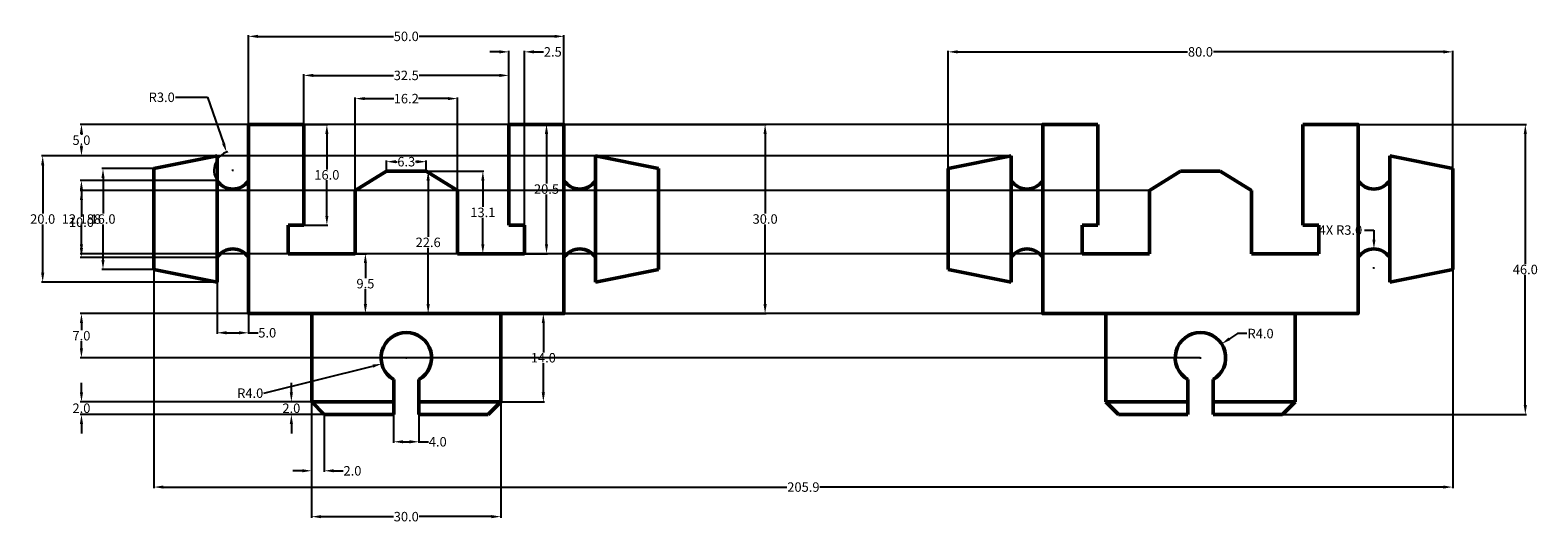
# Model space of a CAD drawing. Units: millimetres. Extents: x 10 to 249, y 5 to 83.
import ezdxf

# ---------------------------------------------------------------- set-up
doc = ezdxf.new("R2010")
doc.units = ezdxf.units.MM
doc.header["$MEASUREMENT"] = 0
doc.layers.add('M-DIMS', color=3, linetype='Continuous', lineweight=25)
doc.layers.add('M-OUTL', color=7, linetype='Continuous', lineweight=50)
doc.styles.get("Standard").update_dxf_attribs({"font": 'arial.ttf'})
doc.dimstyles.get("Standard").update_dxf_attribs({"dimtxt": 1.5, "dimasz": 1.5, "dimexe": 0.18, "dimexo": 0.0625, "dimgap": 0.09, "dimtad": 0, "dimtih": 1, "dimtoh": 1, "dimdec": 1, "dimzin": 0, "dimdsep": 46, "dimtxsty": 'Standard', "dimcen": 0.09, "dimadec": 0, "dimazin": 0, "dimtfac": 1, "dimtdec": 1, "dimtofl": 0, "dimtmove": 0, "dimatfit": 3, "dimfxl": 1, "dimtolj": 1, "dimtzin": 0, "dimarcsym": 0})

# ---------------------------------------------------------------- blocks, each defined once
blk = doc.blocks.new('*D1')
at = {"layer": 'Defpoints', "color": 0, "transparency": 16777216}
for p in [(66.62, 60.41), (72.92, 61.9), (72.92, 60.41)]:
    blk.add_point(p, dxfattribs=at)
at = {"layer": 'M-DIMS', "color": 0, "lineweight": -2, "transparency": 16777216}
for p, q in [((66.62, 60.47), (66.62, 62.08)), ((68.12, 61.9), (68.31, 61.9)), ((71.42, 61.9), (71.23, 61.9)), ((72.92, 60.47), (72.92, 62.08))]:
    blk.add_line(p, q, dxfattribs=at)
at = {"layer": 'M-DIMS', "color": 0, "transparency": 16777216}
for points in [[(68.12, 62.15), (68.12, 61.65), (66.62, 61.9)], [(71.42, 62.15), (71.42, 61.65), (72.92, 61.9)]]:
    blk.add_solid(points, dxfattribs=at)
at = {"layer": 'M-DIMS', "color": 0, "transparency": 16777216, "insert": (69.77, 61.9), "char_height": 1.5, "attachment_point": 5}
blk.add_mtext('\\A1;6.3', dxfattribs=at)
blk = doc.blocks.new('*D2')
at = {"layer": 'Defpoints', "color": 0, "transparency": 16777216}
for p in [(29.77, 60.81), (21.69, 44.81), (29.77, 44.81)]:
    blk.add_point(p, dxfattribs=at)
at = {"layer": 'M-DIMS', "color": 0, "lineweight": -2, "transparency": 16777216}
for p, q in [((29.71, 60.81), (21.51, 60.81)), ((21.69, 59.31), (21.69, 53.67)), ((21.69, 46.31), (21.69, 51.96)), ((29.71, 44.81), (21.51, 44.81))]:
    blk.add_line(p, q, dxfattribs=at)
at = {"layer": 'M-DIMS', "color": 0, "transparency": 16777216}
for points in [[(21.44, 59.31), (21.94, 59.31), (21.69, 60.81)], [(21.44, 46.31), (21.94, 46.31), (21.69, 44.81)]]:
    blk.add_solid(points, dxfattribs=at)
at = {"layer": 'M-DIMS', "color": 0, "transparency": 16777216, "insert": (21.69, 52.81), "char_height": 1.5, "attachment_point": 5}
blk.add_mtext('\\A1;16.0', dxfattribs=at)
blk = doc.blocks.new('*D3')
at = {"layer": 'Defpoints', "color": 0, "transparency": 16777216}
for p in [(39.77, 62.81), (12.13, 42.81), (39.77, 42.81)]:
    blk.add_point(p, dxfattribs=at)
at = {"layer": 'M-DIMS', "color": 0, "lineweight": -2, "transparency": 16777216}
for p, q in [((39.71, 62.81), (11.95, 62.81)), ((12.13, 61.31), (12.13, 53.67)), ((12.13, 44.31), (12.13, 51.96)), ((39.71, 42.81), (11.95, 42.81))]:
    blk.add_line(p, q, dxfattribs=at)
at = {"layer": 'M-DIMS', "color": 0, "transparency": 16777216}
for points in [[(11.88, 61.31), (12.38, 61.31), (12.13, 62.81)], [(11.88, 44.31), (12.38, 44.31), (12.13, 42.81)]]:
    blk.add_solid(points, dxfattribs=at)
at = {"layer": 'M-DIMS', "color": 0, "transparency": 16777216, "insert": (12.13, 52.81), "char_height": 1.5, "attachment_point": 5}
blk.add_mtext('\\A1;20.0', dxfattribs=at)
blk = doc.blocks.new('*D4')
at = {"layer": 'Defpoints', "color": 0, "transparency": 16777216}
for p in [(41.29, 63.4), (42.27, 60.56)]:
    blk.add_point(p, dxfattribs=at)
at = {"layer": 'M-DIMS', "color": 0, "lineweight": -2, "transparency": 16777216}
for p, q in [((33.17, 72.11), (38.25, 72.11)), ((38.25, 72.11), (40.79, 64.81)), ((42.18, 60.56), (42.36, 60.56)), ((42.27, 60.47), (42.27, 60.65))]:
    blk.add_line(p, q, dxfattribs=at)
blk.add_arc((42.27, 60.56), 3, 105.7509, 212.3636, dxfattribs=at)
at = {"layer": 'M-DIMS', "color": 0, "transparency": 16777216}
blk.add_solid([(41.03, 64.9), (40.56, 64.73), (41.29, 63.4)], dxfattribs=at)
at = {"layer": 'M-DIMS', "color": 0, "transparency": 16777216, "insert": (31, 72.11), "char_height": 1.5, "attachment_point": 5}
blk.add_mtext('\\A1;R3.0', dxfattribs=at)
blk = doc.blocks.new('*D5')
at = {"layer": 'Defpoints', "color": 0, "transparency": 16777216}
for p in [(39.77, 42.81), (44.77, 42.81), (44.77, 34.77)]:
    blk.add_point(p, dxfattribs=at)
at = {"layer": 'M-DIMS', "color": 0, "lineweight": -2, "transparency": 16777216}
for p, q in [((39.77, 42.75), (39.77, 34.59)), ((44.77, 42.75), (44.77, 34.59)), ((41.27, 34.77), (43.27, 34.77)), ((44.77, 34.77), (46.27, 34.77))]:
    blk.add_line(p, q, dxfattribs=at)
at = {"layer": 'M-DIMS', "color": 0, "transparency": 16777216}
for points in [[(41.27, 35.02), (41.27, 34.52), (39.77, 34.77)], [(43.27, 35.02), (43.27, 34.52), (44.77, 34.77)]]:
    blk.add_solid(points, dxfattribs=at)
at = {"layer": 'M-DIMS', "color": 0, "transparency": 16777216, "insert": (47.73, 34.77), "char_height": 1.5, "attachment_point": 5}
blk.add_mtext('\\A1;5.0', dxfattribs=at)
blk = doc.blocks.new('*D6')
at = {"layer": 'Defpoints', "color": 0, "transparency": 16777216}
for p in [(65.89, 29.85), (69.77, 30.81)]:
    blk.add_point(p, dxfattribs=at)
at = {"layer": 'M-DIMS', "color": 0, "lineweight": -2, "transparency": 16777216}
for p, q in [((47.2, 25.2), (64.44, 29.48)), ((69.68, 30.81), (69.86, 30.81)), ((69.77, 30.72), (69.77, 30.9))]:
    blk.add_line(p, q, dxfattribs=at)
at = {"layer": 'M-DIMS', "color": 0, "transparency": 16777216}
blk.add_solid([(64.38, 29.73), (64.5, 29.24), (65.89, 29.85)], dxfattribs=at)
at = {"layer": 'M-DIMS', "color": 0, "transparency": 16777216, "insert": (45.03, 25.2), "char_height": 1.5, "attachment_point": 5}
blk.add_mtext('\\A1;R4.0', dxfattribs=at)
blk = doc.blocks.new('*D7')
at = {"layer": 'Defpoints', "color": 0, "transparency": 16777216}
for p in [(54.77, 23.81), (56.77, 21.81), (56.77, 12.89)]:
    blk.add_point(p, dxfattribs=at)
at = {"layer": 'M-DIMS', "color": 0, "lineweight": -2, "transparency": 16777216}
for p, q in [((54.77, 23.75), (54.77, 12.71)), ((56.77, 21.75), (56.77, 12.71)), ((53.27, 12.89), (51.77, 12.89)), ((58.27, 12.89), (59.77, 12.89))]:
    blk.add_line(p, q, dxfattribs=at)
at = {"layer": 'M-DIMS', "color": 0, "transparency": 16777216}
for points in [[(53.27, 13.14), (53.27, 12.64), (54.77, 12.89)], [(58.27, 13.14), (58.27, 12.64), (56.77, 12.89)]]:
    blk.add_solid(points, dxfattribs=at)
at = {"layer": 'M-DIMS', "color": 0, "transparency": 16777216, "insert": (61.24, 12.89), "char_height": 1.5, "attachment_point": 5}
blk.add_mtext('\\A1;2.0', dxfattribs=at)
blk = doc.blocks.new('*D8')
at = {"layer": 'Defpoints', "color": 0, "transparency": 16777216}
for p in [(51.55, 23.81), (54.77, 23.81), (56.77, 21.81)]:
    blk.add_point(p, dxfattribs=at)
at = {"layer": 'M-DIMS', "color": 0, "lineweight": -2, "transparency": 16777216}
for p, q in [((51.55, 25.31), (51.55, 26.81)), ((54.71, 23.81), (51.37, 23.81)), ((56.71, 21.81), (51.37, 21.81)), ((51.55, 20.31), (51.55, 18.81))]:
    blk.add_line(p, q, dxfattribs=at)
at = {"layer": 'M-DIMS', "color": 0, "transparency": 16777216}
for points in [[(51.3, 25.31), (51.8, 25.31), (51.55, 23.81)], [(51.3, 20.31), (51.8, 20.31), (51.55, 21.81)]]:
    blk.add_solid(points, dxfattribs=at)
at = {"layer": 'M-DIMS', "color": 0, "transparency": 16777216, "insert": (51.55, 22.81), "char_height": 1.5, "attachment_point": 5}
blk.add_mtext('\\A1;2.0', dxfattribs=at)
blk = doc.blocks.new('*D9')
at = {"layer": 'Defpoints', "color": 0, "transparency": 16777216}
for p in [(54.77, 23.81), (84.77, 23.81), (84.77, 5.62)]:
    blk.add_point(p, dxfattribs=at)
at = {"layer": 'M-DIMS', "color": 0, "lineweight": -2, "transparency": 16777216}
for p, q in [((54.77, 23.75), (54.77, 5.44)), ((84.77, 23.75), (84.77, 5.44)), ((56.27, 5.62), (67.74, 5.62)), ((83.27, 5.62), (71.81, 5.62))]:
    blk.add_line(p, q, dxfattribs=at)
at = {"layer": 'M-DIMS', "color": 0, "transparency": 16777216}
for points in [[(56.27, 5.87), (56.27, 5.37), (54.77, 5.62)], [(83.27, 5.87), (83.27, 5.37), (84.77, 5.62)]]:
    blk.add_solid(points, dxfattribs=at)
at = {"layer": 'M-DIMS', "color": 0, "transparency": 16777216, "insert": (69.77, 5.62), "char_height": 1.5, "attachment_point": 5}
blk.add_mtext('\\A1;30.0', dxfattribs=at)
blk = doc.blocks.new('*D10')
at = {"layer": 'Defpoints', "color": 0, "transparency": 16777216}
for p in [(67.77, 21.81), (71.77, 21.81), (71.77, 17.49)]:
    blk.add_point(p, dxfattribs=at)
at = {"layer": 'M-DIMS', "color": 0, "lineweight": -2, "transparency": 16777216}
for p, q in [((67.77, 21.75), (67.77, 17.31)), ((71.77, 21.75), (71.77, 17.31)), ((69.27, 17.49), (70.27, 17.49)), ((71.77, 17.49), (73.27, 17.49))]:
    blk.add_line(p, q, dxfattribs=at)
at = {"layer": 'M-DIMS', "color": 0, "transparency": 16777216}
for points in [[(69.27, 17.74), (69.27, 17.24), (67.77, 17.49)], [(70.27, 17.74), (70.27, 17.24), (71.77, 17.49)]]:
    blk.add_solid(points, dxfattribs=at)
at = {"layer": 'M-DIMS', "color": 0, "transparency": 16777216, "insert": (74.76, 17.49), "char_height": 1.5, "attachment_point": 5}
blk.add_mtext('\\A1;4.0', dxfattribs=at)
blk = doc.blocks.new('*D11')
at = {"layer": 'Defpoints', "color": 0, "transparency": 16777216}
for p in [(84.77, 37.81), (91.5, 37.81), (84.77, 23.81)]:
    blk.add_point(p, dxfattribs=at)
at = {"layer": 'M-DIMS', "color": 0, "lineweight": -2, "transparency": 16777216}
for p, q in [((84.84, 37.81), (91.68, 37.81)), ((91.5, 36.31), (91.5, 31.67)), ((91.5, 25.31), (91.5, 29.96)), ((84.84, 23.81), (91.68, 23.81))]:
    blk.add_line(p, q, dxfattribs=at)
at = {"layer": 'M-DIMS', "color": 0, "transparency": 16777216}
for points in [[(91.25, 36.31), (91.75, 36.31), (91.5, 37.81)], [(91.25, 25.31), (91.75, 25.31), (91.5, 23.81)]]:
    blk.add_solid(points, dxfattribs=at)
at = {"layer": 'M-DIMS', "color": 0, "transparency": 16777216, "insert": (91.5, 30.81), "char_height": 1.5, "attachment_point": 5}
blk.add_mtext('\\A1;14.0', dxfattribs=at)
blk = doc.blocks.new('*D12')
at = {"layer": 'Defpoints', "color": 0, "transparency": 16777216}
for p in [(94.77, 67.81), (126.66, 67.81), (94.77, 37.81)]:
    blk.add_point(p, dxfattribs=at)
at = {"layer": 'M-DIMS', "color": 0, "lineweight": -2, "transparency": 16777216}
for p, q in [((94.84, 67.81), (126.84, 67.81)), ((126.66, 66.31), (126.66, 53.67)), ((126.66, 39.31), (126.66, 51.96)), ((94.84, 37.81), (126.84, 37.81))]:
    blk.add_line(p, q, dxfattribs=at)
at = {"layer": 'M-DIMS', "color": 0, "transparency": 16777216}
for points in [[(126.41, 66.31), (126.91, 66.31), (126.66, 67.81)], [(126.41, 39.31), (126.91, 39.31), (126.66, 37.81)]]:
    blk.add_solid(points, dxfattribs=at)
at = {"layer": 'M-DIMS', "color": 0, "transparency": 16777216, "insert": (126.66, 52.81), "char_height": 1.5, "attachment_point": 5}
blk.add_mtext('\\A1;30.0', dxfattribs=at)
blk = doc.blocks.new('*D13')
at = {"layer": 'Defpoints', "color": 0, "transparency": 16777216}
for p in [(94.77, 81.77), (44.77, 67.81), (94.77, 67.81)]:
    blk.add_point(p, dxfattribs=at)
at = {"layer": 'M-DIMS', "color": 0, "lineweight": -2, "transparency": 16777216}
for p, q in [((44.77, 67.87), (44.77, 81.95)), ((46.27, 81.77), (67.74, 81.77)), ((93.27, 81.77), (71.81, 81.77)), ((94.77, 67.87), (94.77, 81.95))]:
    blk.add_line(p, q, dxfattribs=at)
at = {"layer": 'M-DIMS', "color": 0, "transparency": 16777216}
for points in [[(46.27, 82.02), (46.27, 81.52), (44.77, 81.77)], [(93.27, 82.02), (93.27, 81.52), (94.77, 81.77)]]:
    blk.add_solid(points, dxfattribs=at)
at = {"layer": 'M-DIMS', "color": 0, "transparency": 16777216, "insert": (69.77, 81.77), "char_height": 1.5, "attachment_point": 5}
blk.add_mtext('\\A1;50.0', dxfattribs=at)
blk = doc.blocks.new('*D14')
at = {"layer": 'Defpoints', "color": 0, "transparency": 16777216}
for p in [(86.02, 75.58), (53.52, 67.81), (86.02, 67.81)]:
    blk.add_point(p, dxfattribs=at)
at = {"layer": 'M-DIMS', "color": 0, "lineweight": -2, "transparency": 16777216}
for p, q in [((53.52, 67.87), (53.52, 75.76)), ((55.02, 75.58), (67.73, 75.58)), ((84.52, 75.58), (71.82, 75.58)), ((86.02, 67.87), (86.02, 75.76))]:
    blk.add_line(p, q, dxfattribs=at)
at = {"layer": 'M-DIMS', "color": 0, "transparency": 16777216}
for points in [[(55.02, 75.83), (55.02, 75.33), (53.52, 75.58)], [(84.52, 75.83), (84.52, 75.33), (86.02, 75.58)]]:
    blk.add_solid(points, dxfattribs=at)
at = {"layer": 'M-DIMS', "color": 0, "transparency": 16777216, "insert": (69.77, 75.58), "char_height": 1.5, "attachment_point": 5}
blk.add_mtext('\\A1;32.5', dxfattribs=at)
blk = doc.blocks.new('*D15')
at = {"layer": 'Defpoints', "color": 0, "transparency": 16777216}
for p in [(77.87, 71.9), (61.67, 57.31), (77.87, 57.31)]:
    blk.add_point(p, dxfattribs=at)
at = {"layer": 'M-DIMS', "color": 0, "lineweight": -2, "transparency": 16777216}
for p, q in [((61.67, 57.37), (61.67, 72.08)), ((63.17, 71.9), (67.81, 71.9)), ((76.37, 71.9), (71.73, 71.9)), ((77.87, 57.37), (77.87, 72.08))]:
    blk.add_line(p, q, dxfattribs=at)
at = {"layer": 'M-DIMS', "color": 0, "transparency": 16777216}
for points in [[(63.17, 72.15), (63.17, 71.65), (61.67, 71.9)], [(76.37, 72.15), (76.37, 71.65), (77.87, 71.9)]]:
    blk.add_solid(points, dxfattribs=at)
at = {"layer": 'M-DIMS', "color": 0, "transparency": 16777216, "insert": (69.77, 71.9), "char_height": 1.5, "attachment_point": 5}
blk.add_mtext('\\A1;16.2', dxfattribs=at)
blk = doc.blocks.new('*D16')
at = {"layer": 'Defpoints', "color": 0, "transparency": 16777216}
for p in [(53.52, 67.81), (53.52, 51.81), (57.18, 51.81)]:
    blk.add_point(p, dxfattribs=at)
at = {"layer": 'M-DIMS', "color": 0, "lineweight": -2, "transparency": 16777216}
for p, q in [((53.59, 67.81), (57.36, 67.81)), ((57.18, 66.31), (57.18, 60.67)), ((57.18, 53.31), (57.18, 58.96)), ((53.59, 51.81), (57.36, 51.81))]:
    blk.add_line(p, q, dxfattribs=at)
at = {"layer": 'M-DIMS', "color": 0, "transparency": 16777216}
for points in [[(56.93, 66.31), (57.43, 66.31), (57.18, 67.81)], [(56.93, 53.31), (57.43, 53.31), (57.18, 51.81)]]:
    blk.add_solid(points, dxfattribs=at)
at = {"layer": 'M-DIMS', "color": 0, "transparency": 16777216, "insert": (57.18, 59.81), "char_height": 1.5, "attachment_point": 5}
blk.add_mtext('\\A1;16.0', dxfattribs=at)
blk = doc.blocks.new('*D17')
at = {"layer": 'Defpoints', "color": 0, "transparency": 16777216}
for p in [(61.67, 47.31), (61.67, 37.81), (63.29, 37.81)]:
    blk.add_point(p, dxfattribs=at)
at = {"layer": 'M-DIMS', "color": 0, "lineweight": -2, "transparency": 16777216}
for p, q in [((61.74, 47.31), (63.47, 47.31)), ((63.29, 45.81), (63.29, 43.42)), ((63.29, 39.31), (63.29, 41.71)), ((61.74, 37.81), (63.47, 37.81))]:
    blk.add_line(p, q, dxfattribs=at)
at = {"layer": 'M-DIMS', "color": 0, "transparency": 16777216}
for points in [[(63.04, 45.81), (63.54, 45.81), (63.29, 47.31)], [(63.04, 39.31), (63.54, 39.31), (63.29, 37.81)]]:
    blk.add_solid(points, dxfattribs=at)
at = {"layer": 'M-DIMS', "color": 0, "transparency": 16777216, "insert": (63.29, 42.56), "char_height": 1.5, "attachment_point": 5}
blk.add_mtext('\\A1;9.5', dxfattribs=at)
blk = doc.blocks.new('*D18')
at = {"layer": 'Defpoints', "color": 0, "transparency": 16777216}
for p in [(72.92, 60.41), (72.92, 37.81), (73.24, 37.81)]:
    blk.add_point(p, dxfattribs=at)
at = {"layer": 'M-DIMS', "color": 0, "lineweight": -2, "transparency": 16777216}
for p, q in [((72.99, 60.41), (73.42, 60.41)), ((73.24, 58.91), (73.24, 49.97)), ((73.24, 39.31), (73.24, 48.26)), ((72.99, 37.81), (73.42, 37.81))]:
    blk.add_line(p, q, dxfattribs=at)
at = {"layer": 'M-DIMS', "color": 0, "transparency": 16777216}
for points in [[(72.99, 58.91), (73.49, 58.91), (73.24, 60.41)], [(72.99, 39.31), (73.49, 39.31), (73.24, 37.81)]]:
    blk.add_solid(points, dxfattribs=at)
at = {"layer": 'M-DIMS', "color": 0, "transparency": 16777216, "insert": (73.24, 49.11), "char_height": 1.5, "attachment_point": 5}
blk.add_mtext('\\A1;22.6', dxfattribs=at)
blk = doc.blocks.new('*D19')
at = {"layer": 'Defpoints', "color": 0, "transparency": 16777216}
for p in [(72.92, 60.41), (77.87, 47.31), (81.91, 47.31)]:
    blk.add_point(p, dxfattribs=at)
at = {"layer": 'M-DIMS', "color": 0, "lineweight": -2, "transparency": 16777216}
for p, q in [((72.99, 60.41), (82.09, 60.41)), ((81.91, 58.91), (81.91, 54.72)), ((81.91, 48.81), (81.91, 53.01)), ((77.94, 47.31), (82.09, 47.31))]:
    blk.add_line(p, q, dxfattribs=at)
at = {"layer": 'M-DIMS', "color": 0, "transparency": 16777216}
for points in [[(81.66, 58.91), (82.16, 58.91), (81.91, 60.41)], [(81.66, 48.81), (82.16, 48.81), (81.91, 47.31)]]:
    blk.add_solid(points, dxfattribs=at)
at = {"layer": 'M-DIMS', "color": 0, "transparency": 16777216, "insert": (81.91, 53.86), "char_height": 1.5, "attachment_point": 5}
blk.add_mtext('\\A1;13.1', dxfattribs=at)
blk = doc.blocks.new('*D20')
at = {"layer": 'Defpoints', "color": 0, "transparency": 16777216}
for p in [(86.02, 67.81), (92, 67.81), (88.52, 47.31)]:
    blk.add_point(p, dxfattribs=at)
at = {"layer": 'M-DIMS', "color": 0, "lineweight": -2, "transparency": 16777216}
for p, q in [((86.09, 67.81), (92.18, 67.81)), ((92, 66.31), (92, 58.42)), ((92, 48.81), (92, 56.71)), ((88.59, 47.31), (92.18, 47.31))]:
    blk.add_line(p, q, dxfattribs=at)
at = {"layer": 'M-DIMS', "color": 0, "transparency": 16777216}
for points in [[(91.75, 66.31), (92.25, 66.31), (92, 67.81)], [(91.75, 48.81), (92.25, 48.81), (92, 47.31)]]:
    blk.add_solid(points, dxfattribs=at)
at = {"layer": 'M-DIMS', "color": 0, "transparency": 16777216, "insert": (92, 57.56), "char_height": 1.5, "attachment_point": 5}
blk.add_mtext('\\A1;20.5', dxfattribs=at)
blk = doc.blocks.new('MOUNTING-BRACKET-PROFILE')
for p, q in [((-16.25, 30), (-16.25, 14)), ((16.25, 30), (16.25, 14)), ((-40, 23), (-30, 25)), ((-30, 25), (-30, 5)), ((30, 25), (30, 5)), ((40, 23), (30, 25)), ((-40, 23), (-40, 7)), ((-8.1, 19.5), (-3.15, 22.6)), ((-3.15, 22.6), (3.15, 22.6)), ((8.1, 19.5), (3.15, 22.6)), ((40, 23), (40, 7)), ((-8.1, 9.5), (-8.1, 19.5)), ((8.1, 9.5), (8.1, 19.5)), ((-16.25, 14), (-18.75, 14)), ((-18.75, 14), (-18.75, 9.5)), ((16.25, 14), (18.75, 14)), ((18.75, 14), (18.75, 9.5)), ((-18.75, 9.5), (-8.1, 9.5)), ((8.1, 9.5), (18.75, 9.5)), ((-40, 7), (-30, 5)), ((40, 7), (30, 5)), ((-15, -14), (-15, 0)), ((-15, 0), (15, 0)), ((15, 0), (15, -14)), ((-2, -16), (-2, -10.46)), ((2, -16), (2, -10.46)), ((-15, -14), (-2, -14)), ((-13, -16), (-15, -14)), ((2, -14), (15, -14)), ((13, -16), (15, -14)), ((-13, -16), (-2, -16)), ((2, -16), (13, -16))]:
    blk.add_line(p, q)
blk.add_lwpolyline([(16.25, 30), (25, 30), (25, 0), (-25, 0), (-25, 30), (-16.25, 30)])
for centre, radius, start, end in [((-27.5, 22.75), 3, 213.5573, 326.4427), ((27.5, 22.75), 3, 213.5573, 326.4427), ((-27.5, 7.25), 3, 33.5573, 146.4427), ((27.5, 7.25), 3, 33.5573, 146.4427), ((0, -7), 4, 300, 240)]:
    blk.add_arc(centre, radius, start, end)
blk = doc.blocks.new('*D22')
at = {"layer": 'Defpoints', "color": 0, "transparency": 16777216}
for p in [(29.77, 44.81), (235.68, 44.81), (235.68, 10.31)]:
    blk.add_point(p, dxfattribs=at)
at = {"layer": 'M-DIMS', "color": 0, "lineweight": -2, "transparency": 16777216}
for p, q in [((29.77, 44.75), (29.77, 10.13)), ((235.68, 44.75), (235.68, 10.13)), ((31.27, 10.31), (130.09, 10.31)), ((234.18, 10.31), (135.36, 10.31))]:
    blk.add_line(p, q, dxfattribs=at)
at = {"layer": 'M-DIMS', "color": 0, "transparency": 16777216}
for points in [[(31.27, 10.56), (31.27, 10.06), (29.77, 10.31)], [(234.18, 10.56), (234.18, 10.06), (235.68, 10.31)]]:
    blk.add_solid(points, dxfattribs=at)
at = {"layer": 'M-DIMS', "color": 0, "transparency": 16777216, "insert": (132.73, 10.31), "char_height": 1.5, "attachment_point": 5}
blk.add_mtext('\\A1;205.9', dxfattribs=at)
blk = doc.blocks.new('*D23')
at = {"layer": 'Defpoints', "color": 0, "transparency": 16777216}
for p in [(235.68, 79.31), (155.68, 60.81), (235.68, 60.81)]:
    blk.add_point(p, dxfattribs=at)
at = {"layer": 'M-DIMS', "color": 0, "lineweight": -2, "transparency": 16777216}
for p, q in [((155.68, 60.87), (155.68, 79.49)), ((157.18, 79.31), (193.64, 79.31)), ((234.18, 79.31), (197.72, 79.31)), ((235.68, 60.87), (235.68, 79.49))]:
    blk.add_line(p, q, dxfattribs=at)
at = {"layer": 'M-DIMS', "color": 0, "transparency": 16777216}
for points in [[(157.18, 79.56), (157.18, 79.06), (155.68, 79.31)], [(234.18, 79.56), (234.18, 79.06), (235.68, 79.31)]]:
    blk.add_solid(points, dxfattribs=at)
at = {"layer": 'M-DIMS', "color": 0, "transparency": 16777216, "insert": (195.68, 79.31), "char_height": 1.5, "attachment_point": 5}
blk.add_mtext('\\A1;80.0', dxfattribs=at)
blk = doc.blocks.new('*D24')
at = {"layer": 'Defpoints', "color": 0, "transparency": 16777216}
for p in [(18.27, 37.81), (180.68, 37.81), (195.68, 30.81)]:
    blk.add_point(p, dxfattribs=at)
at = {"layer": 'M-DIMS', "color": 0, "lineweight": -2, "transparency": 16777216}
for p, q in [((180.62, 37.81), (18.09, 37.81)), ((18.27, 36.31), (18.27, 35.17)), ((18.27, 32.31), (18.27, 33.46)), ((195.62, 30.81), (18.09, 30.81))]:
    blk.add_line(p, q, dxfattribs=at)
at = {"layer": 'M-DIMS', "color": 0, "transparency": 16777216}
for points in [[(18.02, 36.31), (18.52, 36.31), (18.27, 37.81)], [(18.02, 32.31), (18.52, 32.31), (18.27, 30.81)]]:
    blk.add_solid(points, dxfattribs=at)
at = {"layer": 'M-DIMS', "color": 0, "transparency": 16777216, "insert": (18.27, 34.31), "char_height": 1.5, "attachment_point": 5}
blk.add_mtext('\\A1;7.0', dxfattribs=at)
blk = doc.blocks.new('*D25')
at = {"layer": 'Defpoints', "color": 0, "transparency": 16777216}
for p in [(88.52, 79.31), (86.02, 51.81), (88.52, 51.81)]:
    blk.add_point(p, dxfattribs=at)
at = {"layer": 'M-DIMS', "color": 0, "lineweight": -2, "transparency": 16777216}
for p, q in [((84.52, 79.31), (83.02, 79.31)), ((86.02, 51.87), (86.02, 79.49)), ((88.52, 51.87), (88.52, 79.49)), ((90.02, 79.31), (91.52, 79.31))]:
    blk.add_line(p, q, dxfattribs=at)
at = {"layer": 'M-DIMS', "color": 0, "transparency": 16777216}
for points in [[(84.52, 79.56), (84.52, 79.06), (86.02, 79.31)], [(90.02, 79.56), (90.02, 79.06), (88.52, 79.31)]]:
    blk.add_solid(points, dxfattribs=at)
at = {"layer": 'M-DIMS', "color": 0, "transparency": 16777216, "insert": (93, 79.31), "char_height": 1.5, "attachment_point": 5}
blk.add_mtext('\\A1;2.5', dxfattribs=at)
blk = doc.blocks.new('*D26')
at = {"layer": 'Defpoints', "color": 0, "transparency": 16777216}
for p in [(187.58, 57.31), (18.27, 47.31), (187.58, 47.31)]:
    blk.add_point(p, dxfattribs=at)
at = {"layer": 'M-DIMS', "color": 0, "lineweight": -2, "transparency": 16777216}
for p, q in [((187.52, 57.31), (18.09, 57.31)), ((18.27, 55.81), (18.27, 53.17)), ((18.27, 48.81), (18.27, 51.46)), ((187.52, 47.31), (18.09, 47.31))]:
    blk.add_line(p, q, dxfattribs=at)
at = {"layer": 'M-DIMS', "color": 0, "transparency": 16777216}
for points in [[(18.02, 55.81), (18.52, 55.81), (18.27, 57.31)], [(18.02, 48.81), (18.52, 48.81), (18.27, 47.31)]]:
    blk.add_solid(points, dxfattribs=at)
at = {"layer": 'M-DIMS', "color": 0, "transparency": 16777216, "insert": (18.27, 52.31), "char_height": 1.5, "attachment_point": 5}
blk.add_mtext('\\A1;10.0', dxfattribs=at)
blk = doc.blocks.new('*D27')
at = {"layer": 'Defpoints', "color": 0, "transparency": 16777216}
for p in [(18.274049, 21.811673), (54.774049, 23.811673), (56.774049, 21.811673)]:
    blk.add_point(p, dxfattribs=at)
at = {"layer": 'M-DIMS', "color": 0, "lineweight": -2, "transparency": 16777216}
for p, q in [((18.274049, 25.311673), (18.274049, 26.811673)), ((54.711549, 23.811673), (18.094049, 23.811673)), ((56.711549, 21.811673), (18.094049, 21.811673)), ((18.274049, 20.311673), (18.274049, 18.811673))]:
    blk.add_line(p, q, dxfattribs=at)
at = {"layer": 'M-DIMS', "color": 0, "transparency": 16777216}
for points in [[(18.024049, 25.311673), (18.524049, 25.311673), (18.274049, 23.811673)], [(18.024049, 20.311673), (18.524049, 20.311673), (18.274049, 21.811673)]]:
    blk.add_solid(points, dxfattribs=at)
at = {"layer": 'M-DIMS', "color": 0, "transparency": 16777216, "insert": (18.274049, 22.811673), "char_height": 1.5, "attachment_point": 5}
blk.add_mtext('\\A1;2.0', dxfattribs=at)
blk = doc.blocks.new('*D28')
at = {"layer": 'Defpoints', "color": 0, "transparency": 16777216}
for p in [(18.27, 67.81), (170.68, 67.81), (165.68, 62.81)]:
    blk.add_point(p, dxfattribs=at)
at = {"layer": 'M-DIMS', "color": 0, "lineweight": -2, "transparency": 16777216}
for p, q in [((170.62, 67.81), (18.09, 67.81)), ((18.27, 66.31), (18.27, 66.17)), ((165.62, 62.81), (18.09, 62.81)), ((18.27, 64.31), (18.27, 64.46))]:
    blk.add_line(p, q, dxfattribs=at)
at = {"layer": 'M-DIMS', "color": 0, "transparency": 16777216}
for points in [[(18.02, 66.31), (18.52, 66.31), (18.27, 67.81)], [(18.02, 64.31), (18.52, 64.31), (18.27, 62.81)]]:
    blk.add_solid(points, dxfattribs=at)
at = {"layer": 'M-DIMS', "color": 0, "transparency": 16777216, "insert": (18.27, 65.31), "char_height": 1.5, "attachment_point": 5}
blk.add_mtext('\\A1;5.0', dxfattribs=at)
blk = doc.blocks.new('*D29')
at = {"layer": 'Defpoints', "color": 0, "transparency": 16777216}
for p in [(18.27, 58.91), (39.77, 58.91), (39.77, 46.72)]:
    blk.add_point(p, dxfattribs=at)
at = {"layer": 'M-DIMS', "color": 0, "lineweight": -2, "transparency": 16777216}
for p, q in [((39.71, 58.91), (18.09, 58.91)), ((18.27, 57.41), (18.27, 53.67)), ((18.27, 48.22), (18.27, 51.96)), ((39.71, 46.72), (18.09, 46.72))]:
    blk.add_line(p, q, dxfattribs=at)
at = {"layer": 'M-DIMS', "color": 0, "transparency": 16777216}
for points in [[(18.02, 57.41), (18.52, 57.41), (18.27, 58.91)], [(18.02, 48.22), (18.52, 48.22), (18.27, 46.72)]]:
    blk.add_solid(points, dxfattribs=at)
at = {"layer": 'M-DIMS', "color": 0, "transparency": 16777216, "insert": (18.27, 52.81), "char_height": 1.5, "attachment_point": 5}
blk.add_mtext('\\A1;12.188', dxfattribs=at)
blk = doc.blocks.new('*D30')
at = {"layer": 'Defpoints', "color": 0, "transparency": 16777216}
for p in [(220.68, 67.81), (208.68, 21.81), (247.18, 21.81)]:
    blk.add_point(p, dxfattribs=at)
at = {"layer": 'M-DIMS', "color": 0, "lineweight": -2, "transparency": 16777216}
for p, q in [((220.74, 67.81), (247.36, 67.81)), ((247.18, 66.31), (247.18, 45.67)), ((247.18, 23.31), (247.18, 43.96)), ((208.74, 21.81), (247.36, 21.81))]:
    blk.add_line(p, q, dxfattribs=at)
at = {"layer": 'M-DIMS', "color": 0, "transparency": 16777216}
for points in [[(246.93, 66.31), (247.43, 66.31), (247.18, 67.81)], [(246.93, 23.31), (247.43, 23.31), (247.18, 21.81)]]:
    blk.add_solid(points, dxfattribs=at)
at = {"layer": 'M-DIMS', "color": 0, "transparency": 16777216, "insert": (247.18, 44.81), "char_height": 1.5, "attachment_point": 5}
blk.add_mtext('\\A1;46.0', dxfattribs=at)
blk = doc.blocks.new('*D31')
at = {"layer": 'Defpoints', "color": 0, "transparency": 16777216}
for p in [(223.18, 48.06), (223.18, 45.06)]:
    blk.add_point(p, dxfattribs=at)
at = {"layer": 'M-DIMS', "color": 0, "lineweight": -2, "transparency": 16777216}
for p, q in [((221.68, 51.06), (223.18, 51.06)), ((223.18, 51.06), (223.18, 49.56)), ((223.09, 45.06), (223.27, 45.06)), ((223.18, 44.97), (223.18, 45.15))]:
    blk.add_line(p, q, dxfattribs=at)
at = {"layer": 'M-DIMS', "color": 0, "transparency": 16777216}
blk.add_solid([(223.43, 49.56), (222.93, 49.56), (223.18, 48.06)], dxfattribs=at)
at = {"layer": 'M-DIMS', "color": 0, "transparency": 16777216, "insert": (217.87, 51.06), "char_height": 1.5, "attachment_point": 5}
blk.add_mtext('\\A1;4X R3.0', dxfattribs=at)
blk = doc.blocks.new('*D32')
at = {"layer": 'Defpoints', "color": 0, "transparency": 16777216}
for p in [(199.03, 33), (195.68, 30.81)]:
    blk.add_point(p, dxfattribs=at)
at = {"layer": 'M-DIMS', "color": 0, "lineweight": -2, "transparency": 16777216}
for p, q in [((201.53, 34.65), (200.28, 33.83)), ((203.03, 34.65), (201.53, 34.65)), ((195.59, 30.81), (195.77, 30.81)), ((195.68, 30.72), (195.68, 30.9))]:
    blk.add_line(p, q, dxfattribs=at)
at = {"layer": 'M-DIMS', "color": 0, "transparency": 16777216}
blk.add_solid([(200.14, 34.03), (200.42, 33.62), (199.03, 33)], dxfattribs=at)
at = {"layer": 'M-DIMS', "color": 0, "transparency": 16777216, "insert": (205.21, 34.65), "char_height": 1.5, "attachment_point": 5}
blk.add_mtext('\\A1;R4.0', dxfattribs=at)

msp = doc.modelspace()

# ---------------------------------------------------------------- block references
at = {"layer": 'M-OUTL'}
for p in [(69.774, 37.8117), (195.6794, 37.8117)]:
    msp.add_blockref('MOUNTING-BRACKET-PROFILE', p, dxfattribs=at)

# ---------------------------------------------------------------- dimensions: what is measured, and where the dimension line sits
at = {"layer": 'M-DIMS', "transparency": 33554610}
for base, p1, p2, picture, middle in [((94.774, 81.7707), (44.774, 67.8117), (94.774, 67.8117), '*D13', (69.774, 81.7707)), ((86.024, 75.5761), (53.524, 67.8117), (86.024, 67.8117), '*D14', (69.774, 75.5761)), ((77.874, 71.9011), (61.674, 57.3117), (77.874, 57.3117), '*D15', (69.774, 71.9011)), ((72.924, 61.9022), (66.624, 60.4117), (72.924, 60.4117), '*D1', (69.774, 61.9022)), ((44.774, 34.7685), (39.774, 42.8117), (44.774, 42.8117), '*D5', (47.7269, 34.7685)), ((56.774, 12.8942), (54.774, 23.8117), (56.774, 21.8117), '*D7', (61.2397, 12.8942)), ((84.774, 5.62), (54.774, 23.8117), (84.774, 23.8117), '*D9', (69.774, 5.62)), ((71.774, 17.4907), (67.774, 21.8117), (71.774, 21.8117), '*D10', (74.7571, 17.4907))]:
    dim = msp.add_linear_dim(base=base, p1=p1, p2=p2, dimstyle='Standard', override={"dimclrd": 0, "dimclre": 0, "dimclrt": 0}, dxfattribs=at)
    dim.commit()
    dim.dimension.update_dxf_attribs({"geometry": picture, "text_midpoint": middle})
at = {"layer": 'M-DIMS'}
for base, p1, p2, picture, middle in [((88.524, 79.3117), (86.024, 51.8117), (88.524, 51.8117), '*D25', (92.9979, 79.3117)), ((235.6794, 79.3117), (155.6794, 60.8117), (235.6794, 60.8117), '*D23', (195.6794, 79.3117)), ((235.6794, 10.3117), (29.774, 44.8117), (235.6794, 44.8117), '*D22', (132.7267, 10.3117))]:
    dim = msp.add_linear_dim(base=base, p1=p1, p2=p2, dimstyle='Standard', override={"dimdec": 1, "dimlfac": 1, "dimrnd": 0, "dimzin": 0, "dimdsep": 46, "dimlunit": 2}, dxfattribs=at)
    dim.commit()
    dim.dimension.update_dxf_attribs({"geometry": picture, "text_midpoint": middle})
at = {"layer": 'M-DIMS', "transparency": 33554610}
for center, mpoint, picture, middle in [((42.274, 60.5638), (41.288, 63.3971), '*D4', (31.0036, 72.1126)), ((69.774, 30.8117), (65.8922, 29.8466), '*D6', (47.2032, 25.2002))]:
    dim = msp.add_radius_dim(center=center, mpoint=mpoint, dimstyle='Standard', override={"dimclrd": 0, "dimclre": 0, "dimclrt": 0}, dxfattribs=at)
    dim.commit()
    dim.dimension.update_dxf_attribs({"geometry": picture, "text_midpoint": middle, "dimtype": 164})
at = {"layer": 'M-DIMS'}
for base, p1, p2, override, picture, middle in [((18.274, 67.8117), (165.6794, 62.8117), (170.6794, 67.8117), {"dimdec": 1, "dimlfac": 1, "dimrnd": 0, "dimzin": 0, "dimdsep": 46, "dimlunit": 2}, '*D28', (18.274, 65.3117)), ((247.1794, 21.8117), (220.6794, 67.8117), (208.6794, 21.8117), {"dimdec": 1, "dimlfac": 1, "dimrnd": 0, "dimzin": 0, "dimdsep": 46, "dimlunit": 2}, '*D30', (247.1794, 44.8117)), ((18.274, 58.9055), (39.774, 46.7179), (39.774, 58.9055), {"dimdec": 3, "dimlfac": 1, "dimrnd": 0, "dimzin": 0, "dimdsep": 46, "dimlunit": 2}, '*D29', (18.274, 52.8117)), ((18.274, 47.3117), (187.5794, 57.3117), (187.5794, 47.3117), {"dimdec": 1, "dimlfac": 1, "dimrnd": 0, "dimzin": 0, "dimdsep": 46, "dimlunit": 2}, '*D26', (18.274, 52.3117)), ((18.274, 37.8117), (195.6794, 30.8117), (180.6794, 37.8117), {"dimdec": 1, "dimlfac": 1, "dimrnd": 0, "dimzin": 0, "dimdsep": 46, "dimlunit": 2}, '*D24', (18.274, 34.3117)), ((18.274, 21.8117), (54.774, 23.8117), (56.774, 21.8117), {"dimdec": 1, "dimlfac": 1, "dimrnd": 0, "dimzin": 0, "dimdsep": 46, "dimlunit": 2}, '*D27', (18.274, 22.8117))]:
    dim = msp.add_linear_dim(base=base, p1=p1, p2=p2, angle=90, dimstyle='Standard', override=override, dxfattribs=at)
    dim.commit()
    dim.dimension.update_dxf_attribs({"geometry": picture, "text_midpoint": middle})
at = {"layer": 'M-DIMS', "transparency": 33554610}
for base, p1, p2, picture, middle in [((57.1798, 51.8117), (53.524, 67.8117), (53.524, 51.8117), '*D16', (57.1798, 59.8117)), ((91.9966, 67.8117), (88.524, 47.3117), (86.024, 67.8117), '*D20', (91.9966, 57.5617)), ((126.6577, 67.8117), (94.774, 37.8117), (94.774, 67.8117), '*D12', (126.6577, 52.8117)), ((12.1284, 42.8117), (39.774, 62.8117), (39.774, 42.8117), '*D3', (12.1284, 52.8117)), ((21.6934, 44.8117), (29.774, 60.8117), (29.774, 44.8117), '*D2', (21.6934, 52.8117)), ((73.2371, 37.8117), (72.924, 60.4117), (72.924, 37.8117), '*D18', (73.2371, 49.1117)), ((81.9077, 47.3117), (72.924, 60.4117), (77.874, 47.3117), '*D19', (81.9077, 53.8617)), ((63.2892, 37.8117), (61.674, 47.3117), (61.674, 37.8117), '*D17', (63.2892, 42.5617)), ((91.4954, 37.8117), (84.774, 23.8117), (84.774, 37.8117), '*D11', (91.4954, 30.8117)), ((51.5457, 23.8117), (56.774, 21.8117), (54.774, 23.8117), '*D8', (51.5457, 22.8117))]:
    dim = msp.add_linear_dim(base=base, p1=p1, p2=p2, angle=90, dimstyle='Standard', override={"dimclrd": 0, "dimclre": 0, "dimclrt": 0}, dxfattribs=at)
    dim.commit()
    dim.dimension.update_dxf_attribs({"geometry": picture, "text_midpoint": middle})
at = {"layer": 'M-DIMS'}
dim = msp.add_radius_dim(center=(223.1794, 45.0595), mpoint=(223.179, 48.0595), text='4X <>', dimstyle='Standard', override={"dimdec": 1, "dimlfac": 1, "dimrnd": 0, "dimzin": 0, "dimdsep": 46, "dimlunit": 2}, dxfattribs=at)
dim.commit()
dim.dimension.update_dxf_attribs({"geometry": '*D31', "text_midpoint": (217.8662, 51.0595)})
dim = msp.add_radius_dim(center=(195.6794, 30.8117), mpoint=(199.0254, 33.0035), dimstyle='Standard', override={"dimdec": 1, "dimlfac": 1, "dimrnd": 0, "dimzin": 0, "dimdsep": 46, "dimlunit": 2}, dxfattribs=at)
dim.commit()
dim.dimension.update_dxf_attribs({"geometry": '*D32', "text_midpoint": (205.2056, 34.6474)})

doc.saveas('drawing.dxf')
